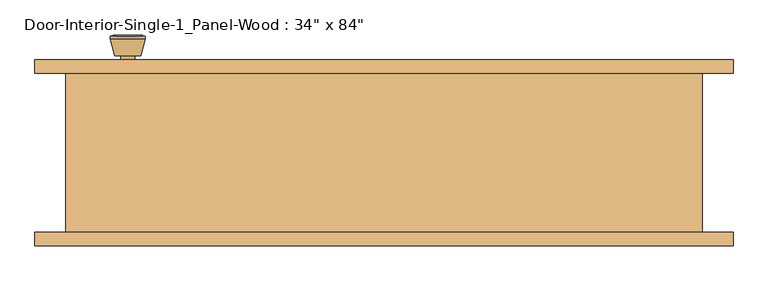
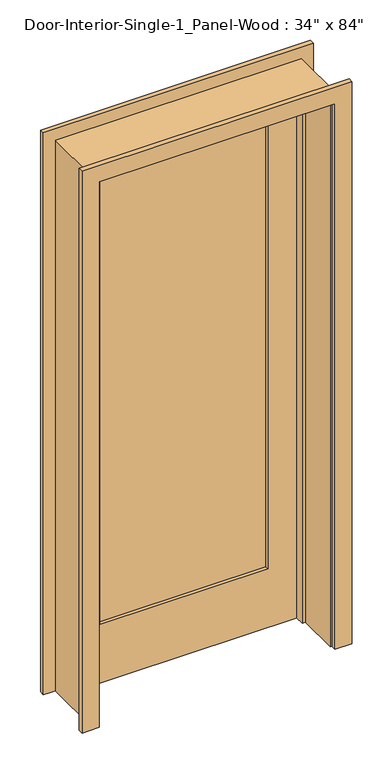
"""IFC4 building model written with IfcOpenShell, lengths in millimetres: door geometry."""

from ifc_helpers import new_model, si_unit, point, frame, frame_2d, origin, place, context, project, spatial, polyline, circle_curve, trimmed, segment, composite_curve, outline, extrude, faceted_brep, source, transform, mapped, element, save
from ifc_brep_helpers import plane_surface, cylinder_surface, revolved_surface, advanced_brep


def door_e2f2f551(model_context):
    return source(origin(), model_context, "Body", "SolidModel", [
        advanced_brep(
        [(-368.3, 70.2, 914.4), (-358.3, 70.2, 914.4), (-378.3, 70.2, 914.4), (-347.8241324, 21.2, 914.4), (-368.3, 21.2, 914.4), (-388.7758676, 21.2, 914.4), (-343.3, 23.0278681, 914.4), (-393.3, 23.0278681, 914.4), (-343.3, 26.4915463, 914.4), (-393.3, 26.4915463, 914.4), (-349.663764, 51.2, 914.4), (-386.936236, 51.2, 914.4), (-358.3, 51.2, 914.4), (-378.3, 51.2, 914.4)],
        [
            (0, 1),
            (1, 2, circle_curve(frame((-368.3, 70.2, 914.4), z_axis=(0.0, 1.0, 0.0), x_axis=(-1.0, 0.0, 0.0)), 10.0)),
            (2, 0),
            (2, 1, circle_curve(frame((-368.3, 70.2, 914.4), z_axis=(0.0, 1.0, 0.0), x_axis=(-1.0, 0.0, 0.0)), 10.0)),
            (3, 4),
            (4, 5),
            (5, 3, circle_curve(frame((-368.3, 21.2, 914.4), z_axis=(0.0, -1.0, 0.0), x_axis=(-1.0, 0.0, 0.0)), 20.4758676)),
            (3, 5, circle_curve(frame((-368.3, 21.2, 914.4), z_axis=(0.0, -1.0, 0.0), x_axis=(-1.0, 0.0, 0.0)), 20.4758676)),
            (6, 3),
            (5, 7),
            (7, 6, circle_curve(frame((-368.3, 23.0278681, 914.4), z_axis=(0.0, -1.0, 0.0), x_axis=(-1.0, 0.0, 0.0)), 25.0)),
            (6, 7, circle_curve(frame((-368.3, 23.0278681, 914.4), z_axis=(0.0, -1.0, 0.0), x_axis=(-1.0, 0.0, 0.0)), 25.0)),
            (8, 6),
            (7, 9),
            (9, 8, circle_curve(frame((-368.3, 26.4915463, 914.4), z_axis=(0.0, -1.0, 0.0), x_axis=(-1.0, 0.0, 0.0)), 25.0)),
            (8, 9, circle_curve(frame((-368.3, 26.4915463, 914.4), z_axis=(0.0, -1.0, 0.0), x_axis=(-1.0, 0.0, 0.0)), 25.0)),
            (10, 8),
            (9, 11),
            (11, 10, circle_curve(frame((-368.3, 51.2, 914.4), z_axis=(0.0, -1.0, 0.0), x_axis=(-1.0, 0.0, 0.0)), 18.636236)),
            (10, 11, circle_curve(frame((-368.3, 51.2, 914.4), z_axis=(0.0, -1.0, 0.0), x_axis=(-1.0, 0.0, 0.0)), 18.636236)),
            (12, 10),
            (11, 13),
            (13, 12, circle_curve(frame((-368.3, 51.2, 914.4), z_axis=(0.0, -1.0, 0.0), x_axis=(-1.0, 0.0, 0.0)), 10.0)),
            (12, 13, circle_curve(frame((-368.3, 51.2, 914.4), z_axis=(0.0, -1.0, 0.0), x_axis=(-1.0, 0.0, 0.0)), 10.0)),
            (1, 12),
            (13, 2),
        ],
        [
            plane_surface(frame((-368.3, 70.2, 914.4), z_axis=(0.0, 1.0, 0.0), x_axis=(-1.0, 0.0, 0.0))),
            plane_surface(frame((-368.3, 21.2, 914.4), z_axis=(0.0, -1.0, 0.0), x_axis=(-1.0, 0.0, 0.0))),
            revolved_surface(polyline([(-388.7758676, 21.2, 914.4), (-393.3, 23.0278681, 914.4)]), (-368.3, 70.2, 914.4), (0.0, 1.0, 0.0)),
            cylinder_surface(frame((-368.3, 70.2, 914.4), z_axis=(0.0, 1.0, 0.0), x_axis=(-1.0, 0.0, 0.0)), 25.0),
            revolved_surface(polyline([(-393.3, 26.4915463, 914.4), (-386.936236, 51.2, 914.4)]), (-368.3, 70.2, 914.4), (0.0, 1.0, 0.0)),
            plane_surface(frame((-368.3, 51.2, 914.4), z_axis=(0.0, 1.0, 0.0), x_axis=(-1.0, 0.0, 0.0))),
            cylinder_surface(frame((-368.3, 70.2, 914.4), z_axis=(0.0, 1.0, 0.0), x_axis=(-1.0, 0.0, 0.0)), 10.0),
        ],
        [
            (0, [[1, 2, 3]]),
            (0, [[-3, 4, -1]]),
            (1, [[5, 6, 7]]),
            (1, [[-6, -5, 8]]),
            (2, [[9, -7, 10, 11]]),
            (2, [[-10, -8, -9, 12]]),
            (3, [[13, -11, 14, 15]]),
            (3, [[-14, -12, -13, 16]]),
            (4, [[17, -15, 18, 19]]),
            (4, [[-18, -16, -17, 20]]),
            (5, [[21, -19, 22, 23]]),
            (5, [[-22, -20, -21, 24]]),
            (6, [[25, -23, 26, -2]]),
            (6, [[-26, -24, -25, -4]]),
        ],
    ),
        extrude(outline(composite_curve([segment(trimmed(circle_curve(frame_2d((914.4, -368.3)), 30.0), [point((914.4, -398.3))], [point((914.4, -338.3))], False, "CARTESIAN"), True, "CONTINUOUS"), segment(trimmed(circle_curve(frame_2d((914.4, -368.3)), 30.0), [point((914.4, -338.3))], [point((914.4, -398.3))], False, "CARTESIAN"), True, "CONTINUOUS")], self_intersect=False)), frame((0.0, 70.2, 0.0), z_axis=(0.0, 1.0, 0.0), x_axis=(0.0, 0.0, 1.0)), (0.0, 0.0, 1.0), 6.0),
        advanced_brep(
        [(-368.3, 117.125, 914.4), (-378.3, 117.125, 914.4), (-358.3, 117.125, 914.4), (-347.8241324, 166.125, 914.4), (-388.7758676, 166.125, 914.4), (-368.3, 166.125, 914.4), (-343.3, 164.2971319, 914.4), (-393.3, 164.2971319, 914.4), (-343.3, 160.8334537, 914.4), (-393.3, 160.8334537, 914.4), (-349.663764, 136.125, 914.4), (-386.936236, 136.125, 914.4), (-358.3, 136.125, 914.4), (-378.3, 136.125, 914.4)],
        [
            (0, 1),
            (1, 2, circle_curve(frame((-368.3, 117.125, 914.4), z_axis=(0.0, -1.0, 0.0), x_axis=(-1.0, 0.0, 0.0)), 10.0)),
            (2, 0),
            (2, 1, circle_curve(frame((-368.3, 117.125, 914.4), z_axis=(0.0, -1.0, 0.0), x_axis=(-1.0, 0.0, 0.0)), 10.0)),
            (3, 4, circle_curve(frame((-368.3, 166.125, 914.4), z_axis=(0.0, 1.0, 0.0), x_axis=(-1.0, 0.0, 0.0)), 20.4758676)),
            (4, 5),
            (5, 3),
            (4, 3, circle_curve(frame((-368.3, 166.125, 914.4), z_axis=(0.0, 1.0, 0.0), x_axis=(-1.0, 0.0, 0.0)), 20.4758676)),
            (6, 7, circle_curve(frame((-368.3, 164.2971319, 914.4), z_axis=(0.0, 1.0, 0.0), x_axis=(-1.0, 0.0, 0.0)), 25.0)),
            (7, 4),
            (3, 6),
            (7, 6, circle_curve(frame((-368.3, 164.2971319, 914.4), z_axis=(0.0, 1.0, 0.0), x_axis=(-1.0, 0.0, 0.0)), 25.0)),
            (8, 9, circle_curve(frame((-368.3, 160.8334537, 914.4), z_axis=(0.0, 1.0, 0.0), x_axis=(-1.0, 0.0, 0.0)), 25.0)),
            (9, 7),
            (6, 8),
            (9, 8, circle_curve(frame((-368.3, 160.8334537, 914.4), z_axis=(0.0, 1.0, 0.0), x_axis=(-1.0, 0.0, 0.0)), 25.0)),
            (10, 11, circle_curve(frame((-368.3, 136.125, 914.4), z_axis=(0.0, 1.0, 0.0), x_axis=(-1.0, 0.0, 0.0)), 18.636236)),
            (11, 9),
            (8, 10),
            (11, 10, circle_curve(frame((-368.3, 136.125, 914.4), z_axis=(0.0, 1.0, 0.0), x_axis=(-1.0, 0.0, 0.0)), 18.636236)),
            (12, 13, circle_curve(frame((-368.3, 136.125, 914.4), z_axis=(0.0, 1.0, 0.0), x_axis=(-1.0, 0.0, 0.0)), 10.0)),
            (13, 11),
            (10, 12),
            (13, 12, circle_curve(frame((-368.3, 136.125, 914.4), z_axis=(0.0, 1.0, 0.0), x_axis=(-1.0, 0.0, 0.0)), 10.0)),
            (1, 13),
            (12, 2),
        ],
        [
            plane_surface(frame((-368.3, 117.125, 914.4), z_axis=(0.0, -1.0, 0.0), x_axis=(-1.0, 0.0, 0.0))),
            plane_surface(frame((-368.3, 166.125, 914.4), z_axis=(0.0, 1.0, 0.0), x_axis=(-1.0, 0.0, 0.0))),
            revolved_surface(polyline([(-388.7758676, 166.125, 914.4), (-393.3, 164.2971319, 914.4)]), (-368.3, 117.125, 914.4), (0.0, -1.0, 0.0)),
            cylinder_surface(frame((-368.3, 117.125, 914.4), z_axis=(0.0, -1.0, 0.0), x_axis=(-1.0, 0.0, 0.0)), 25.0),
            revolved_surface(polyline([(-393.3, 160.8334537, 914.4), (-386.936236, 136.125, 914.4)]), (-368.3, 117.125, 914.4), (0.0, -1.0, 0.0)),
            plane_surface(frame((-368.3, 136.125, 914.4), z_axis=(0.0, -1.0, 0.0), x_axis=(-1.0, 0.0, 0.0))),
            cylinder_surface(frame((-368.3, 117.125, 914.4), z_axis=(0.0, -1.0, 0.0), x_axis=(-1.0, 0.0, 0.0)), 10.0),
        ],
        [
            (0, [[1, 2, 3]]),
            (0, [[-3, 4, -1]]),
            (1, [[5, 6, 7]]),
            (1, [[8, -7, -6]]),
            (2, [[9, 10, -5, 11]]),
            (2, [[12, -11, -8, -10]]),
            (3, [[13, 14, -9, 15]]),
            (3, [[16, -15, -12, -14]]),
            (4, [[17, 18, -13, 19]]),
            (4, [[20, -19, -16, -18]]),
            (5, [[21, 22, -17, 23]]),
            (5, [[24, -23, -20, -22]]),
            (6, [[-2, 25, -21, 26]]),
            (6, [[-4, -26, -24, -25]]),
        ],
    ),
        extrude(outline(composite_curve([segment(trimmed(circle_curve(frame_2d((914.4, -368.3)), 30.0), [point((914.4, -398.3))], [point((914.4, -338.3))], False, "CARTESIAN"), True, "CONTINUOUS"), segment(trimmed(circle_curve(frame_2d((914.4, -368.3)), 30.0), [point((914.4, -338.3))], [point((914.4, -398.3))], False, "CARTESIAN"), True, "CONTINUOUS")], self_intersect=False)), frame((0.0, 111.125, 0.0), z_axis=(0.0, 1.0, 0.0), x_axis=(0.0, 0.0, 1.0)), (0.0, 0.0, 1.0), 6.0),
        faceted_brep([(457.2, 111.125, 0.0), (457.2, -117.475, 0.0), (431.8, -117.475, 0.0), (431.8, 41.275, 0.0), (419.1, 41.275, 0.0), (419.1, 76.2, 0.0), (431.8, 76.2, 0.0), (431.8, 111.125, 0.0), (457.2, 111.125, 2159.0), (457.2, -117.475, 2159.0), (-457.2, -117.475, 2159.0), (-457.2, -117.475, 0.0), (-431.8, -117.475, 0.0), (-431.8, -117.475, 2133.6), (431.8, -117.475, 2133.6), (431.8, 41.275, 2133.6), (-431.8, 41.275, 2133.6), (-431.8, 41.275, 0.0), (-419.1, 41.275, 0.0), (-419.1, 41.275, 2120.9), (419.1, 41.275, 2120.9), (419.1, 76.2, 2120.9), (-419.1, 76.2, 2120.9), (-419.1, 76.2, 0.0), (-431.8, 76.2, 0.0), (-431.8, 76.2, 2133.6), (431.8, 76.2, 2133.6), (431.8, 111.125, 2133.6), (-431.8, 111.125, 2133.6), (-431.8, 111.125, 0.0), (-457.2, 111.125, 0.0), (-457.2, 111.125, 2159.0)], [[[0, 1, 2, 3, 4, 5, 6, 7]], [[1, 0, 8, 9]], [[2, 1, 9, 10, 11, 12, 13, 14]], [[3, 2, 14, 15]], [[4, 3, 15, 16, 17, 18, 19, 20]], [[5, 4, 20, 21]], [[6, 5, 21, 22, 23, 24, 25, 26]], [[7, 6, 26, 27]], [[0, 7, 27, 28, 29, 30, 31, 8]], [[9, 8, 31, 10]], [[15, 14, 13, 16]], [[21, 20, 19, 22]], [[27, 26, 25, 28]], [[30, 29, 24, 23, 18, 17, 12, 11]], [[10, 31, 30, 11]], [[16, 13, 12, 17]], [[22, 19, 18, 23]], [[28, 25, 24, 29]]]),
        extrude(outline(polyline([(2133.6, -431.8), (0.0, -431.8), (0.0, 431.8), (2133.6, 431.8), (2133.6, -431.8)]), holes=[polyline([(2014.5375, -311.15), (2014.5375, 311.15), (231.775, 311.15), (231.775, -311.15), (2014.5375, -311.15)])]), frame((0.0, 76.2, 0.0), z_axis=(0.0, 1.0, 0.0), x_axis=(0.0, 0.0, 1.0)), (0.0, 0.0, 1.0), 34.925),
        extrude(outline(polyline([(311.15, 87.8416667), (-311.15, 87.8416667), (-311.15, 99.4833333), (311.15, 99.4833333), (311.15, 87.8416667)])), frame((0.0, 0.0, 231.775), z_axis=(0.0, 0.0, 1.0), x_axis=(1.0, 0.0, 0.0)), (0.0, 0.0, 1.0), 1782.7625),
        extrude(outline(polyline([(0.0, 438.15), (0.0, 501.65), (2203.45, 501.65), (2203.45, -501.65), (0.0, -501.65), (0.0, -438.15), (2139.95, -438.15), (2139.95, 438.15), (0.0, 438.15)])), frame((0.0, 111.125, 0.0), z_axis=(0.0, 1.0, 0.0), x_axis=(0.0, 0.0, 1.0)), (0.0, 0.0, 1.0), 19.05),
        extrude(outline(polyline([(0.0, 438.15), (0.0, 501.65), (2203.45, 501.65), (2203.45, -501.65), (0.0, -501.65), (0.0, -438.15), (2139.95, -438.15), (2139.95, 438.15), (0.0, 438.15)])), frame((0.0, -136.525, 0.0), z_axis=(0.0, 1.0, 0.0), x_axis=(0.0, 0.0, 1.0)), (0.0, 0.0, 1.0), 19.05),
    ])


if __name__ == "__main__":
    model = new_model("IFC4")
    model_context = context("Model", 3, world=origin())
    ifc_project = project(units=[si_unit("LENGTHUNIT", "METRE", prefix="MILLI")], contexts=[model_context])
    site = spatial("IfcSite", under=ifc_project)
    building = spatial("IfcBuilding", under=site)
    placement = place(None, origin())
    door_shape = door_e2f2f551(model_context)
    element("IfcDoor", 1, ObjectType="Door-Interior-Single-1_Panel-Wood : 34\" x 84\"", at=placement, inside=building, context=model_context, shape_type="MappedRepresentation", body=[
        mapped(door_shape, transform((0.0, 0.0, 0.0), x_axis=(1.0, 0.0, 0.0), y_axis=(0.0, 1.0, 0.0), z_axis=(0.0, 0.0, 1.0))),
    ])
    save(model, "model.ifc")

# Revit data of these elements
# Type "Door-Interior-Single-1_Panel-Wood : 34\" x 84\""
#   Type Mark = "9"
#   Assembly Code = "C1020300"
#   Analytic Construction = "Wooden"
#   Top Rail = 0' - 4 11/16"
#   Thickness = 0' - 1 3/8"
#   Thermal Resistance (R) = 2.5876 (h·ft²·°F)/BTU
#   Swing Angle [instance default] = 90.00°
#   Stiles = 0' - 4 3/4"
#   Rough Width = 3' - 0"
#   Rough Height = 7' - 1"
#   Height = 7' - 0"
#   Width = 2' - 10"
#   Heat Transfer Coefficient (U) = 0.3865 BTU/(h·ft²·°F)
#   Bottom Rail = 0' - 9 1/8"
#   Trim Material = Cherry
#   Panel Material = Cherry
#   Frame Material = Cherry
#   Door Handle Material = Aluminum
#   Visual Light Transmittance = 0
#   Solar Heat Gain Coefficient = 0
#   Wall Closure = (empty or 0)
#   Function = (empty or 0)
# Element 1 (IfcDoor, "Door-Interior-Single-1_Panel-Wood : 34\" x 84\"")
#   Materials on its faces: "Cherry", "Aluminum"
# Materials
#   "Cherry": class "Wood", colour RGB 226 177 128, transparency 0, Description = "Prunus Serotina", Cost = 0
#   "Aluminum": class "Metal", colour RGB 247 247 247, transparency 0, Description = "Aluminum 6061", Cost = 0
